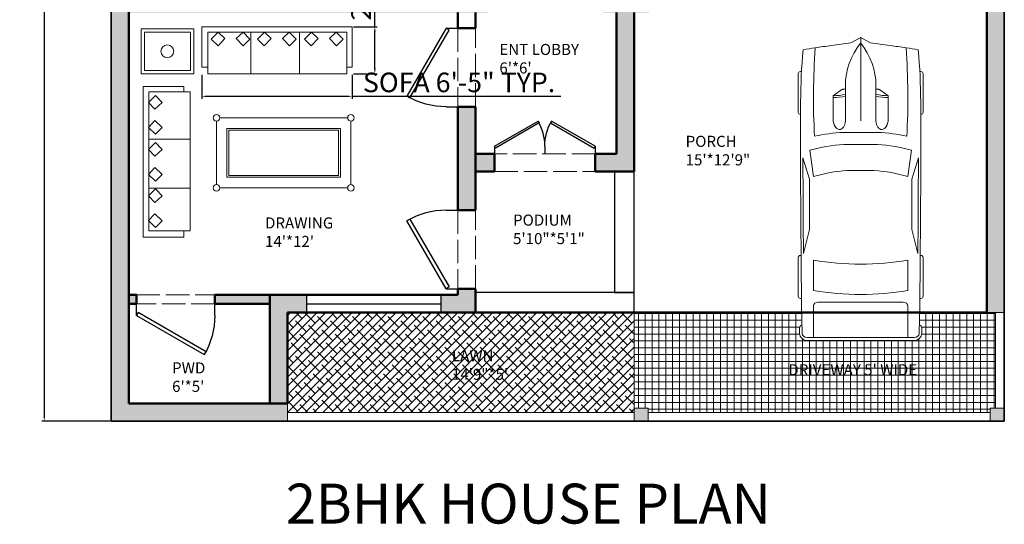
# Model space of a CAD drawing. Units: inches. Extents: x 2101 to 2698, y 3451 to 4160.
# Tile 1 of 3: x 2101 to 2604, y 3451 to 3709. Entities that reach past the tile are written whole.
import ezdxf

# ---------------------------------------------------------------- set-up
doc = ezdxf.new("R2010")
doc.units = ezdxf.units.IN
doc.linetypes.add('ACAD_ISO02W100', pattern=[15, 12, -3])
for name, color, linetype, lineweight in [('A-ANNO-DIMS', 40, 'Continuous', 18), ('A-ANNO-TEXT', 40, 'Continuous', 25), ('A-AREA-IDEN', 40, 'Continuous', 18), ('A-FLOR', 7, 'Continuous', 25), ('A-FLOR-PATT', 252, 'Continuous', 13), ('A-SITE-VEHI', 8, 'Continuous', 18), ('A-WALL-OVHD', 150, 'ACAD_ISO02W100', 18), ('A-WALL-PATT', 150, 'Continuous', 13), ('C-PROP', 7, 'Continuous', 35), ('C-SITE-PVMT', 8, 'Continuous', 18), ('DOOR', 52, 'Continuous', 25), ('FURNITURE', 132, 'Continuous', 18), ('WALL', 150, 'Continuous', 50), ('WIN', 210, 'Continuous', 25)]:
    doc.layers.add(name, color=color, linetype=linetype, lineweight=lineweight)
doc.styles.get("Standard").update_dxf_attribs({"font": 'arial.ttf'})
doc.dimstyles.new('ISO-25', dxfattribs={"dimtxt": 10, "dimasz": 2.5, "dimexe": 1.25, "dimexo": 0.625, "dimtad": 1, "dimdec": 0, "dimlunit": 4, "dimtxsty": 'Standard', "dimcen": 2.5, "dimadec": 0, "dimazin": 0, "dimtfac": 1, "dimtdec": 0, "dimtmove": 0, "dimatfit": 3, "dimfxl": 1, "dimarcsym": 0})

# ---------------------------------------------------------------- blocks, each defined once
blk = doc.blocks.new('*U2')
for p, q in [((0, 0), (0, -6)), ((40, 0), (40, -6))]:
    blk.add_line(p, q)
blk.add_lwpolyline([(0, 0), (34.64, 20), (35.52, 18.48), (0.87, -1.52)], close=True)
blk.add_arc((0, 0), 40, 0, 30)
blk = doc.blocks.new('*U6')
for p, q in [((21.1, 37.41), (21.1, 36.83)), ((46.55, 38.89), (22.35, 38.89)), ((47.8, 37.39), (47.8, 37.41)), ((135.45, 37.07), (135.45, 37.41)), ((136.7, 38.89), (160.9, 38.89)), ((162.15, 37.41), (162.15, 36.77)), ((70.03, 31.54), (86.41, 29.35)), ((87.99, 31.87), (74.76, 35.92)), ((134.31, 35.6), (119.29, 31.78)), ((186.47, -33.5), (186.47, 33.5)), ((188.4, -32.76), (188.4, 32.76)), ((138.42, 29.35), (157.25, 29.35)), ((164.52, 26.39), (164.52, -26.39)), ((186.47, 29.35), (167.01, 29.35)), ((32.27, 11.63), (36.13, 17.17)), ((36.13, 17.17), (50.94, 17.17)), ((29.77, 9.51), (51.68, 9.51)), ((32.12, 9.51), (32.12, 11.15)), ((58.92, -10.77), (58.92, 10.77)), ((66.55, -10.53), (66.55, 10.53)), ((82.74, 8.5), (82.74, -8.5)), ((186.47, -10.53), (186.47, 10.53)), ((3.27, 6.13), (0.1, 0.41)), ((0, 0), (51.68, 0)), ((0.1, -0.41), (3.27, -6.13)), ((29.77, -9.51), (51.68, -9.51)), ((32.12, -9.51), (32.12, -11.15)), ((32.27, -11.63), (36.13, -17.17)), ((36.13, -17.17), (50.94, -17.17)), ((86.41, -29.35), (70.03, -31.54)), ((157.25, -29.35), (138.42, -29.35)), ((167.01, -29.35), (186.47, -29.35)), ((87.99, -31.87), (74.76, -35.92)), ((134.31, -35.6), (119.29, -31.78)), ((21.1, -37.41), (21.1, -36.83)), ((46.55, -38.89), (22.35, -38.89)), ((47.8, -37.39), (47.8, -37.41)), ((135.45, -37.07), (135.45, -37.41)), ((136.7, -38.89), (160.9, -38.89)), ((162.15, -37.41), (162.15, -36.77))]:
    blk.add_line(p, q)
for centre, major_axis, ratio, start_param, end_param in [((41.19, -490.86), (0, 528.23), 0.842304, 0.00281, 0.075598), ((22.35, 37.41), (0, -1.48), 0.842304, 3.141593, 4.712389), ((64.48, -10555.62), (0, 10593.03), 0.842304, -0.013397, 0.002797), ((46.55, 37.41), (0, 1.48), 0.842304, -1.570796, 0), ((136.7, 37.41), (0, -1.48), 0.842304, 3.141593, 4.712389), ((160.9, 37.41), (0, 1.48), 0.842304, -1.570796, 0), ((180.63, 35.84), (0, 2.22), 0.842304, -0.013017, 1.249894), ((64.48, -10556.36), (0, 10595.31), 0.842304, -0.013397, -0.013017), ((183.98, 32.76), (0, -5.25), 0.842304, 1.570796, 3.128196), ((266.03, -27.52), (0, 313.31), 0.842304, 1.367076, 1.39176), ((135.29, 5.39), (0, 81.77), 0.842304, 1.245306, 1.50788), ((64.48, -10555.62), (0, -10591.55), 0.842304, 3.133765, 3.140441), ((95.79, -3666.35), (0, -3698.24), 0.842304, 3.134049, 3.144098), ((183.98, 33.5), (0, -2.96), 0.842304, 1.570796, 3.128196), ((259.18, -27.52), (0, -305.3), 0.842304, 4.528606, 4.561838), ((37.47, -593.96), (0, -623.33), 0.842304, 3.096046, 3.200911), ((134.4, 5.39), (0, -89.78), 0.842304, 4.449482, 4.652344), ((149.6, 2.8), (0, -79.58), 0.842304, 4.372215, 4.640744), ((17.08, 0), (0, 147.02), 0.842304, 4.511394, 4.913384), ((35.91, 0), (0, 147.02), 0.842304, 4.511394, 4.913384), ((167.01, 26.39), (0, 2.96), 0.842304, 0, 1.570796), ((-204.49, 52.4), (0, -250.96), 0.842304, 1.385369, 1.434372), ((13.04, 17.01), (0, 27.42), 0.842304, 4.435146, 4.718221), ((14.2, 17.01), (0, 27.42), 0.842304, 4.435146, 4.718221), ((50.79, 13.34), (6.34, -0.36), 0.603834, -1.395552, 1.581315), ((29.77, -46.66), (0, 56.17), 0.842304, 0, 0.590319), ((32.75, 11.15), (0, 0.74), 0.842304, 0.879714, 1.570796), ((0.62, 0), (0, -0.74), 0.842304, 4.131459, 5.293319), ((-204.49, -52.4), (0, 250.96), 0.842304, -1.434372, -1.385369), ((29.77, 46.66), (0, 56.17), 0.842304, 2.551274, 3.141593), ((32.75, -11.15), (0, -0.74), 0.842304, 4.712389, 5.403472), ((13.04, -17.01), (0, -27.42), 0.842304, 1.564964, 1.848039), ((14.2, -17.01), (0, -27.42), 0.842304, 1.564964, 1.848039), ((134.4, -5.39), (0, -89.78), 0.842304, -1.510751, -1.307889), ((135.29, -5.39), (0, -81.77), 0.842304, -1.50788, -1.245306), ((149.6, -2.8), (0, -79.58), 0.842304, -1.499151, -1.230623), ((259.18, 27.52), (0, 305.3), 0.842304, 1.721348, 1.754579), ((266.03, 27.52), (0, 313.31), 0.842304, 1.749832, 1.774517), ((37.47, 593.96), (0, -623.33), 0.842304, -0.059319, 0.045547), ((167.01, -26.39), (0, -2.96), 0.842304, 4.712389, 6.283185), ((41.19, 490.86), (0, -528.23), 0.842304, -0.075598, -0.00281), ((64.48, 10555.62), (0, 10593.03), 0.842304, 3.138796, 3.15499), ((64.48, 10555.62), (0, -10591.55), 0.842304, 0.001152, 0.007828), ((95.79, 3666.35), (0, -3698.24), 0.842304, -0.002505, 0.007544), ((180.63, -35.84), (0, -2.22), 0.842304, -1.249894, 0.013017), ((183.98, -33.5), (0, 2.96), 0.842304, 3.15499, 4.712389), ((183.98, -32.76), (0, -5.25), 0.842304, 0.013397, 1.570796), ((22.35, -37.41), (0, 1.48), 0.842304, 1.570796, 3.141593), ((46.55, -37.41), (0, -1.48), 0.842304, 0, 1.570796), ((136.7, -37.41), (0, -1.48), 0.842304, -1.570796, 0), ((160.9, -37.41), (0, 1.48), 0.842304, 3.141593, 4.712389), ((64.48, 10556.36), (0, 10595.31), 0.842304, 3.15461, 3.15499)]:
    blk.add_ellipse(centre, major_axis=major_axis, ratio=ratio, start_param=start_param, end_param=end_param)
at = {"extrusion": (0, 0, -1)}
blk.add_ellipse((50.79, -13.34), major_axis=(6.34, 0.36), ratio=0.603834, start_param=-1.395552, end_param=1.581315, dxfattribs=at)
blk = doc.blocks.new('*D8')
at = {"layer": 'A-ANNO-DIMS', "color": 0, "lineweight": -2, "transparency": 16777216}
for p, q in [((2147.02, 4103.85), (2112.19, 4103.85)), ((2113.44, 4101.35), (2113.44, 3506.35)), ((2147.02, 3503.85), (2112.19, 3503.85))]:
    blk.add_line(p, q, dxfattribs=at)
at = {"layer": 'A-ANNO-DIMS', "color": 0, "lineweight": 100, "transparency": 16777216}
for points in [[(2113.03, 4101.35), (2113.86, 4101.35), (2113.44, 4103.85)], [(2113.03, 3506.35), (2113.86, 3506.35), (2113.44, 3503.85)]]:
    blk.add_solid(points, dxfattribs=at)
at = {"layer": 'Defpoints', "color": 0, "lineweight": 100, "transparency": 16777216}
for p in [(2147.64, 4103.85), (2113.44, 3503.85), (2147.64, 3503.85)]:
    blk.add_point(p, dxfattribs=at)
at = {"layer": 'A-ANNO-DIMS', "color": 0, "transparency": 16777216, "insert": (2107.71, 3803.85), "char_height": 10, "attachment_point": 5, "rotation": 90}
blk.add_mtext("50'", dxfattribs=at)
blk = doc.blocks.new('SOFA-THREE-SEAT-CUSHIONED')
for p, q in [((0, 3.26), (0, 23.95)), ((0, 23.95), (76.85, 23.95)), ((24.98, 21.14), (24.98, 0)), ((49.98, 21.14), (49.98, 0)), ((76.85, 23.95), (76.85, 3.26)), ((3.17, 3.26), (0, 3.26)), ((3.17, 3.26), (3.17, 3.26)), ((76.85, 3.26), (74.12, 3.26))]:
    blk.add_line(p, q)
for points in [[(3.17, 21.14), (74.12, 21.14), (74.12, 0), (3.17, 0)], [(8.4, 21.27), (11.83, 17.94), (8.31, 14.3), (4.87, 17.63)], [(21.06, 21.27), (17.62, 17.94), (21.15, 14.3), (24.59, 17.63)], [(32.03, 21.27), (35.47, 17.94), (31.94, 14.3), (28.5, 17.63)], [(44.69, 21.27), (41.25, 17.94), (44.78, 14.3), (48.22, 17.63)], [(56, 21.27), (59.44, 17.94), (55.91, 14.3), (52.47, 17.63)], [(68.66, 21.27), (65.22, 17.94), (68.75, 14.3), (72.19, 17.63)]]:
    blk.add_lwpolyline(points, close=True)
blk = doc.blocks.new('*D21')
at = {"layer": 'A-ANNO-DIMS', "color": 0, "lineweight": -2, "transparency": 16777216}
for p, q in [((2193.86, 3680.57), (2193.86, 3668.41)), ((2270.71, 3680.57), (2270.71, 3668.41)), ((2196.36, 3669.66), (2268.21, 3669.66)), ((2270.71, 3669.66), (2377.29, 3669.66))]:
    blk.add_line(p, q, dxfattribs=at)
at = {"layer": 'A-ANNO-DIMS', "color": 0, "lineweight": 100, "transparency": 16777216}
for points in [[(2196.36, 3670.08), (2196.36, 3669.25), (2193.86, 3669.66)], [(2268.21, 3670.08), (2268.21, 3669.25), (2270.71, 3669.66)]]:
    blk.add_solid(points, dxfattribs=at)
at = {"layer": 'Defpoints', "color": 0, "lineweight": 100, "transparency": 16777216}
for p in [(2193.86, 3681.19), (2270.71, 3681.19), (2270.71, 3669.66)]:
    blk.add_point(p, dxfattribs=at)
at = {"layer": 'A-ANNO-DIMS', "color": 0, "transparency": 16777216, "insert": (2325.25, 3675.46), "char_height": 10, "attachment_point": 5}
blk.add_mtext('SOFA 6\'-5" TYP.', dxfattribs=at)
blk = doc.blocks.new('*D22')
at = {"layer": 'A-ANNO-DIMS', "color": 0, "lineweight": -2, "transparency": 16777216}
for p, q in [((2282.24, 3705.14), (2282.24, 3770.01)), ((2271.34, 3705.14), (2283.49, 3705.14)), ((2282.24, 3683.69), (2282.24, 3702.64)), ((2271.34, 3681.19), (2283.49, 3681.19))]:
    blk.add_line(p, q, dxfattribs=at)
at = {"layer": 'A-ANNO-DIMS', "color": 0, "lineweight": 100, "transparency": 16777216}
for points in [[(2281.82, 3702.64), (2282.66, 3702.64), (2282.24, 3705.14)], [(2281.82, 3683.69), (2282.66, 3683.69), (2282.24, 3681.19)]]:
    blk.add_solid(points, dxfattribs=at)
at = {"layer": 'Defpoints', "color": 0, "lineweight": 100, "transparency": 16777216}
for p in [(2270.71, 3705.14), (2282.24, 3705.14), (2270.71, 3681.19)]:
    blk.add_point(p, dxfattribs=at)
at = {"layer": 'A-ANNO-DIMS', "color": 0, "transparency": 16777216, "insert": (2276.51, 3738.83), "char_height": 10, "attachment_point": 5, "rotation": 90}
blk.add_mtext('2\'-0" TYP.', dxfattribs=at)

msp = doc.modelspace()

# ---------------------------------------------------------------- hatches: boundary and pattern name
at = {"layer": 'A-FLOR-PATT'}
h = msp.add_hatch(dxfattribs=at)
h.set_pattern_fill('ANSI38', color=256)
h.paths.add_polyline_path([(2599.14, 3862.35), (2594.64, 3862.35), (2539.14, 3862.35), (2539.14, 3814.35), (2594.64, 3814.35), (2599.14, 3814.35)])
h.paths.add_polyline_path([(2414.64, 3559.35), (2333.64, 3559.35), (2237.64, 3559.35), (2237.64, 3512.85), (2237.64, 3508.35), (2414.64, 3508.35), (2414.64, 3510.57)])
h = msp.add_hatch(dxfattribs=at)
h.set_pattern_fill('NET', color=256, scale=1.1)
h.paths.add_polyline_path([(2560.27, 3552.87), (2560.54, 3552.78), (2560.78, 3552.65), (2561, 3552.49), (2561.18, 3552.31), (2561.33, 3552.1), (2561.44, 3551.88), (2561.5, 3551.64), (2561.52, 3551.4), (2561.5, 3550.01), (2561.47, 3548.62), (2561.4, 3548), (2561.2, 3547.39), (2560.88, 3546.83), (2560.45, 3546.32), (2559.92, 3545.88), (2559.31, 3545.52), (2558.63, 3545.26), (2557.91, 3545.1), (2557.17, 3545.04), (2503.42, 3545.04), (2502.68, 3545.1), (2501.96, 3545.26), (2501.29, 3545.52), (2500.68, 3545.88), (2500.15, 3546.32), (2499.72, 3546.83), (2499.39, 3547.39), (2499.19, 3548), (2499.12, 3548.62), (2499.1, 3550.01), (2499.08, 3551.4), (2499.1, 3551.64), (2499.16, 3551.88), (2499.27, 3552.1), (2499.41, 3552.31), (2499.6, 3552.49), (2499.81, 3552.65), (2500.06, 3552.78), (2500.32, 3552.88), (2500.25, 3557.61), (2500.23, 3559.35), (2414.64, 3559.35), (2414.64, 3510.57), (2421.88, 3510.57), (2421.88, 3508.35), (2596.41, 3508.35), (2596.41, 3510.57), (2599.14, 3510.57), (2599.14, 3559.35), (2560.37, 3559.35)])
at = {"layer": 'A-WALL-PATT'}
h = msp.add_hatch(color=256, dxfattribs=at)
h.dxf.hatch_style = 1
h.paths.add_polyline_path([(2156.64, 4103.85), (2147.64, 4103.85), (2147.64, 4099.35), (2156.64, 4099.35)])
h.paths.add_polyline_path([(2163.74, 4034.85), (2156.64, 4034.85), (2156.64, 4025.85), (2163.74, 4025.85)])
h.paths.add_polyline_path([(2333.64, 3874.35), (2333.64, 3879.64), (2324.64, 3879.64), (2324.64, 3874.35), (2213.91, 3874.35), (2213.91, 3865.35), (2333.64, 3865.35)])
h.paths.add_polyline_path([(2333.64, 3977.85), (2324.64, 3977.85), (2324.64, 3934.78), (2324.64, 3919.64), (2333.64, 3919.64)])
h.paths.add_polyline_path([(2161.58, 3874.35), (2156.64, 3874.35), (2156.64, 3865.35), (2161.58, 3865.35)])
h.paths.add_polyline_path([(2541.41, 3935.85), (2414.64, 3935.85), (2414.64, 3938.14), (2405.64, 3938.14), (2405.64, 3926.85), (2541.41, 3926.85)])
h.paths.add_polyline_path([(2594.64, 3935.85), (2581.41, 3935.85), (2581.41, 3926.85), (2594.64, 3926.85)])
h.paths.add_polyline_path([(2539.14, 3926.85), (2530.14, 3926.85), (2530.14, 3862.35), (2556.24, 3862.35), (2556.24, 3866.85), (2539.14, 3866.85)])
h.paths.add_polyline_path([(2599.14, 3866.85), (2594.64, 3866.85), (2578.65, 3866.85), (2578.65, 3862.35), (2594.64, 3862.35), (2599.14, 3862.35)])
h.paths.add_polyline_path([(2414.64, 3885.48), (2405.64, 3885.48), (2405.64, 3809.85), (2414.64, 3809.85), (2414.64, 3818.85), (2414.64, 3842.85)])
h.paths.add_polyline_path([(2530.14, 3818.85), (2414.64, 3818.85), (2414.64, 3809.85), (2450.64, 3809.85), (2530.14, 3809.85)])
h.paths.add_polyline_path([(2414.64, 3809.85), (2405.64, 3809.85), (2405.64, 3721.35), (2414.64, 3721.35), (2414.64, 3725.85)])
h.paths.add_polyline_path([(2603.64, 3814.35), (2599.14, 3814.35), (2594.64, 3814.35), (2594.64, 3559.35), (2603.64, 3559.35)])
h.paths.add_polyline_path([(2594.64, 3814.35), (2530.14, 3814.35), (2530.14, 3809.85), (2594.64, 3809.85)])
h = msp.add_hatch(color=256, dxfattribs=at)
h.dxf.hatch_style = 1
h.paths.add_polyline_path([(2603.64, 3814.35), (2599.14, 3814.35), (2594.64, 3814.35), (2594.64, 3559.35), (2603.64, 3559.35)])
h = msp.add_hatch(color=256, dxfattribs=at)
h.dxf.hatch_style = 1
h.paths.add_polyline_path([(2228.64, 3568.35), (2200.53, 3568.35), (2200.53, 3563.85), (2228.64, 3563.85)])
h.paths.add_polyline_path([(2339.85, 3721.35), (2333.64, 3721.35), (2225.64, 3721.35), (2225.64, 3712.35), (2324.64, 3712.35), (2339.85, 3712.35)])
h.paths.add_polyline_path([(2225.64, 3721.35), (2156.64, 3721.35), (2156.64, 3712.35), (2225.64, 3712.35)])
h.paths.add_polyline_path([(2225.64, 3790), (2216.64, 3790), (2216.64, 3785.85), (2201.25, 3785.85), (2201.25, 3781.35), (2225.64, 3781.35)])
h.paths.add_polyline_path([(2225.64, 3781.35), (2221.14, 3781.35), (2221.14, 3764.71), (2225.64, 3764.71)])
h.paths.add_polyline_path([(2175.48, 3785.85), (2156.64, 3785.85), (2156.64, 3781.35), (2175.48, 3781.35)])
h.paths.add_polyline_path([(2414.64, 3809.85), (2405.64, 3809.85), (2405.64, 3721.35), (2414.64, 3721.35), (2414.64, 3725.85)])
h.paths.add_polyline_path([(2422.2, 3721.35), (2398.52, 3721.35), (2398.52, 3712.35), (2422.2, 3712.35)])
h = msp.add_hatch(color=256, dxfattribs=at)
h.dxf.hatch_style = 1
h.paths.add_polyline_path([(2247.32, 3568.35), (2228.64, 3568.35), (2228.64, 3559.35), (2228.64, 3512.85), (2237.64, 3512.85), (2237.64, 3559.35), (2247.32, 3559.35)], flags=17)
h.paths.add_polyline_path([(2228.64, 3568.35), (2200.53, 3568.35), (2200.53, 3563.85), (2228.64, 3563.85)], flags=17)
h.paths.add_polyline_path([(2333.64, 3569.5), (2333.64, 3571.5), (2324.64, 3571.5), (2324.64, 3568.35), (2316.02, 3568.35), (2316.02, 3559.35), (2333.64, 3559.35)])
h.paths.add_polyline_path([(2237.64, 3512.85), (2228.64, 3512.85), (2156.64, 3512.85), (2156.64, 3721.35), (2147.64, 3721.35), (2147.64, 3503.85), (2237.64, 3503.85)])
h.paths.add_polyline_path([(2237.64, 3559.35), (2247.32, 3559.35), (2247.32, 3568.35), (2228.64, 3568.35), (2228.64, 3563.85), (2228.64, 3559.35), (2228.64, 3512.85), (2237.64, 3512.85)], flags=17)
h = msp.add_hatch(color=256, dxfattribs=at)
h.dxf.hatch_style = 1
h.paths.add_polyline_path([(2247.32, 3568.35), (2228.64, 3568.35), (2228.64, 3559.35), (2228.64, 3512.85), (2237.64, 3512.85), (2237.64, 3559.35), (2247.32, 3559.35)])
h.paths.add_polyline_path([(2228.64, 3568.35), (2200.53, 3568.35), (2200.53, 3563.85), (2228.64, 3563.85)])
h.paths.add_polyline_path([(2333.64, 3569.5), (2333.64, 3571.5), (2324.64, 3571.5), (2324.64, 3568.35), (2316.02, 3568.35), (2316.02, 3559.35), (2333.64, 3559.35)])
h.paths.add_polyline_path([(2333.64, 3664.35), (2324.64, 3664.35), (2324.64, 3611.5), (2333.64, 3611.5)])
h.paths.add_polyline_path([(2343.31, 3640.35), (2333.64, 3640.35), (2333.64, 3631.35), (2343.31, 3631.35)])
h.paths.add_polyline_path([(2414.64, 3712.35), (2405.64, 3712.35), (2405.64, 3640.35), (2394.74, 3640.35), (2394.74, 3631.35), (2414.64, 3631.35)])
h = msp.add_hatch(color=256, dxfattribs=at)
h.dxf.hatch_style = 1
h.paths.add_polyline_path([(2333.64, 3571.5), (2324.64, 3571.5), (2324.64, 3568.35), (2316.02, 3568.35), (2316.02, 3559.35), (2333.64, 3559.35)])
h.paths.add_polyline_path([(2237.64, 3559.35), (2247.32, 3559.35), (2247.32, 3568.35), (2228.64, 3568.35), (2228.64, 3559.35), (2228.64, 3512.85), (2237.64, 3512.85)])
h.paths.add_polyline_path([(2421.88, 3510.57), (2414.64, 3510.57), (2414.64, 3503.85), (2421.88, 3503.85)])
h.paths.add_polyline_path([(2603.64, 3510.57), (2596.41, 3510.57), (2596.41, 3503.85), (2603.64, 3503.85)])
h.paths.add_polyline_path([(2333.64, 3664.35), (2324.64, 3664.35), (2324.64, 3611.5), (2333.64, 3611.5)])
h.paths.add_polyline_path([(2414.64, 3712.35), (2405.64, 3712.35), (2405.64, 3640.35), (2394.74, 3640.35), (2394.74, 3631.35), (2414.64, 3631.35)])
h.paths.add_polyline_path([(2343.31, 3640.35), (2333.64, 3640.35), (2333.64, 3631.35), (2343.31, 3631.35)])
h = msp.add_hatch(color=256, dxfattribs=at)
h.dxf.hatch_style = 1
h.paths.add_polyline_path([(2160.53, 3568.35), (2156.64, 3568.35), (2156.64, 3563.85), (2160.53, 3563.85)])
h.paths.add_polyline_path([(2228.64, 3568.35), (2200.53, 3568.35), (2200.53, 3563.85), (2228.64, 3563.85)])
h = msp.add_hatch(color=256, dxfattribs=at)
h.dxf.hatch_style = 1
h.paths.add_polyline_path([(2228.64, 3568.35), (2200.53, 3568.35), (2200.53, 3563.85), (2228.64, 3563.85)])
h = msp.add_hatch(color=256, dxfattribs=at)
h.dxf.hatch_style = 1
h.paths.add_polyline_path([(2421.88, 3510.57), (2414.64, 3510.57), (2414.64, 3503.85), (2421.88, 3503.85)])
h.paths.add_polyline_path([(2603.64, 3510.57), (2596.41, 3510.57), (2596.41, 3503.85), (2603.64, 3503.85)])
h.paths.add_polyline_path([(2228.64, 3568.35), (2200.53, 3568.35), (2200.53, 3563.85), (2228.64, 3563.85)])

# ---------------------------------------------------------------- linework, layer by layer
at = {"layer": 'A-FLOR'}
for points in [[(2414.64, 3631.35), (2404.6, 3631.35), (2404.6, 3569.5), (2414.64, 3569.5)], [(2333.64, 3559.35), (2414.65, 3559.35), (2414.65, 3569.5), (2333.64, 3569.5)]]:
    msp.add_lwpolyline(points, close=True, dxfattribs=at)
at = {"layer": 'A-WALL-OVHD'}
for points in [[(2324.64, 3664.35), (2333.64, 3664.35), (2333.64, 3704.35), (2324.64, 3704.35)], [(2343.31, 3631.35), (2394.74, 3631.35), (2394.74, 3640.35), (2343.31, 3640.35)], [(2324.64, 3571.5), (2333.64, 3571.5), (2333.64, 3611.5), (2324.64, 3611.5)], [(2160.53, 3568.35), (2200.53, 3568.35), (2200.53, 3563.85), (2160.53, 3563.85)]]:
    msp.add_lwpolyline(points, close=True, dxfattribs=at)
at = {"layer": 'C-PROP'}
for p, q in [((2147.64, 3503.85), (2147.64, 4103.85)), ((2603.64, 4103.85), (2603.64, 3503.85)), ((2603.64, 3503.85), (2147.64, 3503.85))]:
    msp.add_line(p, q, dxfattribs=at)
at = {"layer": 'C-SITE-PVMT'}
for p, q in [((2414.64, 3508.35), (2414.64, 3559.35)), ((2594.64, 3559.35), (2603.64, 3559.35)), ((2599.14, 3559.35), (2599.14, 3510.57)), ((2237.64, 3512.85), (2237.64, 3503.85)), ((2237.64, 3508.35), (2414.64, 3508.35)), ((2237.64, 3508.35), (2414.64, 3508.35)), ((2421.88, 3508.35), (2596.41, 3508.35))]:
    msp.add_line(p, q, dxfattribs=at)
for points in [[(2414.64, 3503.85), (2421.88, 3503.85), (2421.88, 3510.57), (2414.64, 3510.57)], [(2596.41, 3503.85), (2603.64, 3503.85), (2603.64, 3510.57), (2596.41, 3510.57)]]:
    msp.add_lwpolyline(points, close=True, dxfattribs=at)
at = {"layer": 'FURNITURE'}
for points in [[(2162.84, 3704.15), (2189.77, 3704.15), (2189.77, 3681.11), (2162.84, 3681.11)], [(2164.55, 3702.44), (2188.06, 3702.44), (2188.06, 3682.82), (2164.55, 3682.82)], [(2164.55, 3702.44), (2188.06, 3702.44), (2188.06, 3682.82), (2164.55, 3682.82)], [(2206.74, 3653.31), (2264.66, 3653.31), (2264.66, 3628.33), (2206.74, 3628.33)], [(2207.74, 3652.31), (2263.66, 3652.31), (2263.66, 3629.33), (2207.74, 3629.33)]]:
    msp.add_lwpolyline(points, close=True, dxfattribs=at)
for points in [[(2201.37, 3624.61), (2201.37, 3657.03)], [(2203.01, 3658.67), (2268.39, 3658.67)], [(2270.03, 3657.03), (2270.03, 3624.61)], [(2268.39, 3622.97), (2203.01, 3622.97)]]:
    msp.add_lwpolyline(points, dxfattribs=at)
for centre, radius in [((2176.3, 3692.63), 3.25), ((2201.37, 3658.67), 1.64), ((2270.03, 3658.67), 1.64), ((2201.37, 3622.97), 1.64), ((2270.03, 3622.97), 1.64)]:
    msp.add_circle(centre, radius, dxfattribs=at)
at = {"layer": 'WALL'}
for p, q in [((2156.64, 3512.85), (2156.64, 4099.35)), ((2594.64, 3814.35), (2594.64, 3559.35)), ((2324.64, 3712.35), (2324.64, 3704.35)), ((2333.64, 3712.35), (2333.64, 3704.35)), ((2333.64, 3712.35), (2333.64, 3704.35)), ((2405.64, 3640.35), (2405.64, 3712.35)), ((2414.64, 3631.35), (2414.64, 3712.35)), ((2324.64, 3664.35), (2324.64, 3611.5)), ((2333.64, 3664.35), (2333.64, 3640.35)), ((2333.64, 3664.35), (2333.64, 3611.5)), ((2333.64, 3640.35), (2343.31, 3640.35)), ((2394.74, 3640.35), (2405.64, 3640.35)), ((2333.64, 3631.35), (2343.31, 3631.35)), ((2394.74, 3631.35), (2414.64, 3631.35)), ((2324.64, 3571.5), (2324.64, 3568.35)), ((2333.64, 3571.5), (2333.64, 3559.35)), ((2160.53, 3568.35), (2156.64, 3568.35)), ((2324.64, 3568.35), (2200.53, 3568.35)), ((2228.64, 3559.35), (2228.64, 3568.35)), ((2156.64, 3563.85), (2160.53, 3563.85)), ((2200.53, 3563.85), (2228.64, 3563.85)), ((2228.64, 3559.35), (2228.64, 3512.85)), ((2333.64, 3559.35), (2237.64, 3559.35)), ((2237.64, 3559.35), (2237.64, 3512.85)), ((2333.64, 3559.35), (2594.64, 3559.35)), ((2237.64, 3512.85), (2156.64, 3512.85))]:
    msp.add_line(p, q, dxfattribs=at)
for points in [[(2333.64, 3704.35), (2324.64, 3704.35)], [(2324.64, 3664.35), (2333.64, 3664.35)], [(2343.31, 3631.35), (2343.31, 3640.35)], [(2394.74, 3640.35), (2394.74, 3631.35)], [(2333.64, 3611.5), (2324.64, 3611.5)], [(2324.64, 3571.5), (2333.64, 3571.5)], [(2160.53, 3568.35), (2160.53, 3563.85)], [(2200.53, 3563.85), (2200.53, 3568.35)]]:
    msp.add_lwpolyline(points, dxfattribs=at)
at = {"layer": 'WIN'}
msp.add_line((2247.32, 3563.85), (2316.02, 3563.85), dxfattribs=at)
msp.add_lwpolyline([(2247.32, 3559.35), (2316.02, 3559.35), (2316.02, 3568.35), (2247.32, 3568.35)], close=True, dxfattribs=at)

# ---------------------------------------------------------------- block references
at = {"layer": 'A-SITE-VEHI', "xscale": 0.8203604116824129, "yscale": 0.8203604116824129, "zscale": 0.8203604116824129, "rotation": 270}
msp.add_blockref('*U6', (2530.3, 3699.6), dxfattribs=at)
at = {"layer": 'DOOR', "xscale": -1}
for p, rotation in [((2318.64, 3704.35), 90), ((2160.53, 3557.85), 180)]:
    msp.add_blockref('*U2', p, dxfattribs=dict(at, rotation=rotation))
at = {"layer": 'DOOR', "yscale": 0.6428675240530186, "zscale": 0.6428675240530186}
for p, xscale in [((2343.31, 3644.2), 0.6428675240530186), ((2394.74, 3644.2), -0.6428675240530186)]:
    msp.add_blockref('*U2', p, dxfattribs=dict(at, xscale=xscale))
at = {"layer": 'DOOR', "rotation": 90}
msp.add_blockref('*U2', (2318.64, 3571.5), dxfattribs=at)
at = {"layer": 'FURNITURE'}
msp.add_blockref('SOFA-THREE-SEAT-CUSHIONED', (2193.86, 3681.19), dxfattribs=at)
at = {"layer": 'FURNITURE', "rotation": 90.00000000000556}
msp.add_blockref('SOFA-THREE-SEAT-CUSHIONED', (2187.91, 3597.81), dxfattribs=at)

# ---------------------------------------------------------------- texts
at = {"layer": 'A-ANNO-TEXT', "insert": (2236.76, 3472.02), "char_height": 20.365, "attachment_point": 1}
msp.add_mtext_dynamic_manual_height_columns('2BHK HOUSE PLAN', width=3624.0333, gutter_width=101.83, heights=[0], dxfattribs=at)
at = {"layer": 'A-AREA-IDEN', "attachment_point": 1}
for s, insert, char_height in [("ENT LOBBY\\P6'*6'", (2345.84, 3696.39), 5.657), ('PORCH\\P15\'*12\'9"', (2440.93, 3649.5), 5.657), ("DRAWING\\P14'*12'", (2226.16, 3607.87), 5.657), ('PODIUM\\P5\'10"*5\'1"', (2352.81, 3609.32), 5.657), ('LAWN\\P14\'9"*5\'', (2321.6, 3540.09), 5.657), ("PWD\\P6'*5'", (2178.72, 3533.92), 5.657), ("DRIVEWAY 5' WIDE", (2493.37, 3532.98), 5.6568)]:
    msp.add_mtext_dynamic_manual_height_columns(s, width=91.5864, gutter_width=28.28, heights=[0], dxfattribs=dict(at, insert=insert, char_height=char_height))

# ---------------------------------------------------------------- dimensions: what is measured, and where the dimension line sits
at = {"layer": 'A-ANNO-DIMS'}
dim = msp.add_linear_dim(base=(2113.44, 3503.85), p1=(2147.64, 4103.85), p2=(2147.64, 3503.85), angle=90, dimstyle='ISO-25', override={"dimclrd": 0, "dimclre": 0, "dimclrt": 0}, dxfattribs=at)
dim.commit()
dim.dimension.update_dxf_attribs({"geometry": '*D8', "text_midpoint": (2107.71, 3803.85)})
dim = msp.add_linear_dim(base=(2282.241, 3705.1377), p1=(2270.7131, 3681.1925), p2=(2270.7131, 3705.1377), angle=90, text='<> TYP.', dimstyle='ISO-25', override={"dimdec": 1, "dimlfac": 1, "dimrnd": 0, "dimzin": 1, "dimdsep": 46, "dimlunit": 4, "dimfrac": 2}, dxfattribs=at)
dim.commit()
dim.dimension.update_dxf_attribs({"geometry": '*D22', "text_midpoint": (2276.5103, 3738.8255)})
dim = msp.add_linear_dim(base=(2270.7131, 3669.6646), p1=(2193.8603, 3681.1925), p2=(2270.7131, 3681.1925), text='SOFA <> TYP.', dimstyle='ISO-25', override={"dimdec": 1, "dimlfac": 1, "dimrnd": 0, "dimzin": 1, "dimdsep": 46, "dimlunit": 4, "dimfrac": 2}, dxfattribs=at)
dim.commit()
dim.dimension.update_dxf_attribs({"geometry": '*D21', "text_midpoint": (2325.2501, 3675.4635)})

doc.saveas('drawing.dxf')
